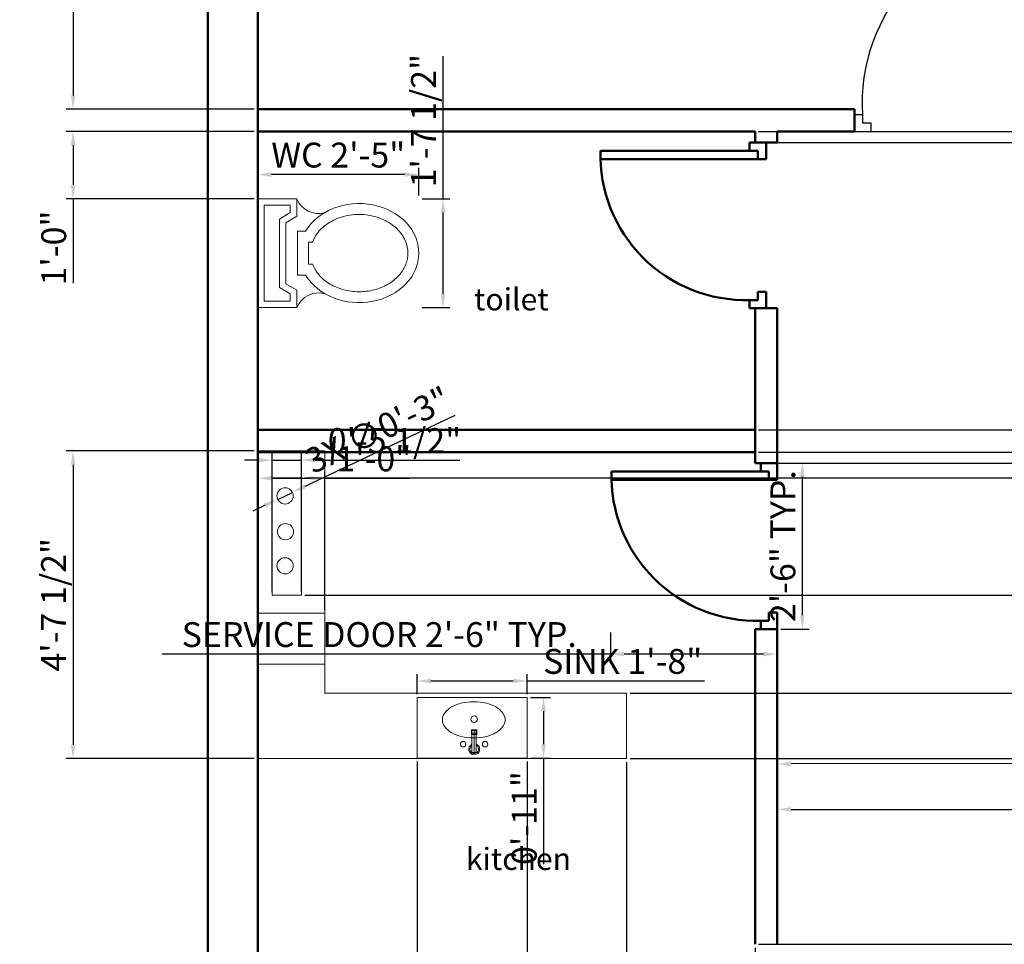
# Model space of a CAD drawing. Units: inches. Extents: x 1253 to 1645, y 2180 to 2698.
# Tile 2 of 5: x 1253 to 1431, y 2363 to 2531. Entities that reach past the tile are written whole.
import ezdxf

# ---------------------------------------------------------------- set-up
doc = ezdxf.new("R2010")
doc.units = ezdxf.units.IN
for name, color, linetype, lineweight in [('A-ANNO-DIMS', 2, 'Continuous', 18), ('A-AREA-IDEN', 7, 'Continuous', 25), ('A-DOOR', 4, 'Continuous', 25), ('A-FLOR-FIXT', 9, 'Continuous', 18), ('wall', 7, 'Continuous', 50)]:
    doc.layers.add(name, color=color, linetype=linetype, lineweight=lineweight)
doc.styles.get("Standard").update_dxf_attribs({"font": 'arial.ttf'})
doc.dimstyles.new('ISO-25', dxfattribs={"dimtxt": 4.5, "dimasz": 2.5, "dimexe": 1.25, "dimexo": 0.625, "dimtad": 1, "dimdec": 1, "dimlunit": 3, "dimtxsty": 'Standard', "dimcen": 4.5, "dimadec": 0, "dimazin": 0, "dimtfac": 1, "dimtdec": 1, "dimtmove": 0, "dimatfit": 3, "dimfxl": 1, "dimarcsym": 0})

# ---------------------------------------------------------------- blocks, each defined once
blk = doc.blocks.new('new block')
for p, q in [((1.5, 1.5), (1.5, 30)), ((3, 0), (3, 30)), ((0, 3), (0, 0)), ((1.5, 3), (0, 3)), ((1.5, 1.5), (1.5, 3)), ((28.5, 1.5), (28.5, 3)), ((28.5, 3), (30, 3)), ((30, 3), (30, 0)), ((0, 0), (3, 0)), ((3, 1.5), (1.5, 1.5)), ((3, 0), (3, 1.5)), ((27, 0), (27, 1.5)), ((27, 1.5), (28.5, 1.5)), ((30, 0), (27, 0))]:
    blk.add_line(p, q)
blk.add_arc((2.25, 3.75), 26.26, 358.3634, 91.6366)
blk = doc.blocks.new('2.6door')
at = {"layer": 'wall'}
blk.add_blockref('new block', (0, 0), dxfattribs=at)
blk = doc.blocks.new('A$C7C8779AE')
for p, q in [((0, 0.7405), (0, 0.5605)), ((0.5, 0.7405), (0, 0.7405)), ((0.5, 0.5605), (0.5, 0.7405)), ((0.47, 0.7105), (0.03, 0.7105)), ((0.03, 0.7105), (0.03, 0.5905)), ((0.47, 0.5905), (0.47, 0.7105)), ((0.093, 0.6405), (0.063, 0.5905)), ((0.093, 0.6405), (0.407, 0.6405)), ((0.437, 0.5905), (0.407, 0.6405)), ((0.03, 0.5905), (0.063, 0.5905)), ((0.11, 0.6105), (0.08, 0.5605)), ((0.11, 0.6105), (0.39, 0.6105)), ((0.42, 0.5605), (0.39, 0.6105)), ((0.437, 0.5905), (0.47, 0.5905)), ((0, 0.5605), (0.08, 0.5605)), ((0.1497, 0.557), (0.1497, 0.5203)), ((0.1497, 0.557), (0.3514, 0.557)), ((0.3514, 0.557), (0.3514, 0.5203)), ((0.42, 0.5605), (0.5, 0.5605)), ((0.1997, 0.507), (0.1997, 0.4879)), ((0.1997, 0.507), (0.3014, 0.507)), ((0.3014, 0.507), (0.3014, 0.4879))]:
    blk.add_line(p, q)
for centre, start, end in [((-0.0386, 0.4613), 344.642, 68.7339), ((0.5386, 0.4613), 111.2661, 195.358)]:
    blk.add_arc(centre, 0.1064, start, end)
blk.add_ellipse((0.2506, 0.2744), major_axis=(0, 0.2744), ratio=0.828948, start_param=0.459479, end_param=5.823706)
blk.add_open_spline([(0.1997, 0.4879), (0.1697, 0.474), (0.1642, 0.4702), (0.1512, 0.4602), (0.1438, 0.4535), (0.1298, 0.4388), (0.1233, 0.4306), (0.1111, 0.4131), (0.1055, 0.4037), (0.0956, 0.3838), (0.0912, 0.3733), (0.0838, 0.3516), (0.0808, 0.3403), (0.0762, 0.3172), (0.0746, 0.3055), (0.073, 0.2817), (0.0729, 0.2698), (0.0743, 0.246), (0.0758, 0.2342), (0.0801, 0.2111), (0.0831, 0.1998), (0.0903, 0.1779), (0.0945, 0.1673), (0.1043, 0.1473), (0.1098, 0.1378), (0.1218, 0.12), (0.1283, 0.1118), (0.1421, 0.0968), (0.1494, 0.09), (0.1646, 0.078), (0.1725, 0.0728), (0.1887, 0.064), (0.1969, 0.0603), (0.2137, 0.0547), (0.2222, 0.0527), (0.2392, 0.0502), (0.2478, 0.0498), (0.2664, 0.0505), (0.2764, 0.052), (0.2963, 0.0573), (0.3061, 0.061), (0.3253, 0.0707), (0.3346, 0.0766), (0.3525, 0.0906), (0.3611, 0.0987), (0.3771, 0.1169), (0.3845, 0.127), (0.3978, 0.1488), (0.4037, 0.1605), (0.4137, 0.1853), (0.4178, 0.1983), (0.424, 0.2251), (0.4261, 0.2389), (0.4282, 0.2668), (0.4283, 0.2809), (0.4262, 0.3088), (0.4241, 0.3226), (0.418, 0.3495), (0.414, 0.3625), (0.404, 0.3873), (0.3982, 0.3991), (0.385, 0.421), (0.3776, 0.4311), (0.3617, 0.4494), (0.3531, 0.4575), (0.3382, 0.4693), (0.3321, 0.4736), (0.3014, 0.4879)], degree=3, knots=[0.459479, 0.459479, 0.459479, 0.459479, 0.567422, 0.567422, 0.720865, 0.720865, 0.874307, 0.874307, 1.02775, 1.02775, 1.181192, 1.181192, 1.334635, 1.334635, 1.488077, 1.488077, 1.64152, 1.64152, 1.794963, 1.794963, 1.948405, 1.948405, 2.101848, 2.101848, 2.25529, 2.25529, 2.408733, 2.408733, 2.562175, 2.562175, 2.715618, 2.715618, 2.86906, 2.86906, 3.022503, 3.022503, 3.175946, 3.175946, 3.356457, 3.356457, 3.536968, 3.536968, 3.717479, 3.717479, 3.89799, 3.89799, 4.078501, 4.078501, 4.259012, 4.259012, 4.439523, 4.439523, 4.620035, 4.620035, 4.800546, 4.800546, 4.981057, 4.981057, 5.161568, 5.161568, 5.342079, 5.342079, 5.52259, 5.52259, 5.703101, 5.703101, 5.823706, 5.823706, 5.823706, 5.823706])
blk = doc.blocks.new('A$C50A015BB')
for p, q in [((0, 0.55), (1, 0.55)), ((0, 0.55), (0, 0)), ((1, 0.55), (1, 0)), ((0.4985, 0.5), (0.5385, 0.5)), ((0.4985, 0.5), (0.4985, 0.3)), ((0.5185, 0.5), (0.5185, 0.3)), ((0.5385, 0.5), (0.5385, 0.3)), ((0.4935, 0.335), (0.4935, 0.295)), ((0.4935, 0.335), (0.5435, 0.335)), ((0.4935, 0.295), (0.5435, 0.295)), ((0.4985, 0.325), (0.5385, 0.325)), ((0.4985, 0.3), (0.5385, 0.3)), ((0.5435, 0.335), (0.5435, 0.295)), ((0, 0), (1, 0)), ((0, 0), (1, 0))]:
    blk.add_line(p, q)
for centre, radius in [((0.4185, 0.424), 0.025), ((0.6185, 0.424), 0.025), ((0.5185, 0.1981), 0.0298)]:
    blk.add_circle(centre, radius)
for centre, radius, start, end in [((0.5201, 0.4703), 0.0497, 291.74253, 244.23308), ((0.5201, 0.4703), 0.0397, 297.63203, 237.02558), ((0.5157, -0.1225), 0.4906, 90, 103.48533), ((0.5157, -0.1225), 0.4906, 76.51467, 90), ((0.4185, 0.1397), 0.2081, 120.06859, 144.41781), ((0.4772, 0.0383), 0.3252, 103.48533, 120.06859), ((0.5543, 0.0383), 0.3252, 59.93141, 76.51467), ((0.613, 0.1397), 0.2081, 35.58219, 59.93141), ((0.3299, 0.2031), 0.0991, 144.41781, 180), ((0.3299, 0.2031), 0.0991, 180, 215.58219), ((0.7016, 0.2031), 0.0991, 0, 35.58219), ((0.7016, 0.2031), 0.0991, 324.41781, 0), ((0.4185, 0.2665), 0.2081, 215.58219, 239.93141), ((0.613, 0.2665), 0.2081, 300.06859, 324.41781), ((0.4772, 0.3679), 0.3252, 239.93141, 256.51467), ((0.5157, 0.5288), 0.4906, 256.51467, 270), ((0.5157, 0.5288), 0.4906, 270, 283.48533), ((0.5543, 0.3679), 0.3252, 283.48533, 300.06859)]:
    blk.add_arc(centre, radius, start, end)
blk = doc.blocks.new('DOOR-SWING-36IN')
for p, q in [((1.5, 1.5), (1.5, 37.5)), ((3, 1.5), (3, 37.5)), ((0, 3), (0, 0)), ((1.5, 3), (0, 3)), ((1.5, 1.5), (1.5, 3)), ((34.5, 1.5), (34.5, 3)), ((34.5, 3), (36, 3)), ((36, 3), (36, 0)), ((3, 1.5), (1.5, 1.5)), ((3, 0), (3, 1.5)), ((33, 0), (33, 1.5)), ((33, 1.5), (34.5, 1.5)), ((0, 0), (3, 0)), ((36, 0), (33, 0))]:
    blk.add_line(p, q)
blk.add_arc((2.25, 5.18), 32.32, 356.1244, 91.3295)
blk = doc.blocks.new('*D20')
at = {"layer": 'A-ANNO-DIMS', "color": 0, "lineweight": -2, "transparency": 16777216}
for p, q in [((1359.74, 2419.72), (1359.74, 2414.57)), ((1389.94, 2419.72), (1389.94, 2414.57)), ((1359.74, 2415.82), (1278.63, 2415.82)), ((1387.44, 2415.82), (1362.24, 2415.82))]:
    blk.add_line(p, q, dxfattribs=at)
at = {"layer": 'A-ANNO-DIMS', "color": 0, "transparency": 16777216}
for points in [[(1362.24, 2416.23), (1362.24, 2415.4), (1359.74, 2415.82)], [(1387.44, 2416.23), (1387.44, 2415.4), (1389.94, 2415.82)]]:
    blk.add_solid(points, dxfattribs=at)
at = {"layer": 'Defpoints', "color": 0, "transparency": 16777216}
for p in [(1359.74, 2420.35), (1389.94, 2420.35), (1359.74, 2415.82)]:
    blk.add_point(p, dxfattribs=at)
at = {"layer": 'A-ANNO-DIMS', "color": 0, "transparency": 16777216, "insert": (1317.93, 2418.77), "char_height": 4.5, "attachment_point": 5}
blk.add_mtext('SERVICE DOOR 2\'-6" TYP.', dxfattribs=at)
blk = doc.blocks.new('*D21')
at = {"layer": 'A-ANNO-DIMS', "color": 0, "lineweight": -2, "transparency": 16777216}
for p, q in [((1390.57, 2450.35), (1395.72, 2450.35)), ((1394.47, 2447.85), (1394.47, 2422.85)), ((1390.57, 2420.35), (1395.72, 2420.35))]:
    blk.add_line(p, q, dxfattribs=at)
at = {"layer": 'A-ANNO-DIMS', "color": 0, "transparency": 16777216}
for points in [[(1394.06, 2447.85), (1394.89, 2447.85), (1394.47, 2450.35)], [(1394.06, 2422.85), (1394.89, 2422.85), (1394.47, 2420.35)]]:
    blk.add_solid(points, dxfattribs=at)
at = {"layer": 'Defpoints', "color": 0, "transparency": 16777216}
for p in [(1389.94, 2450.35), (1389.94, 2420.35), (1394.47, 2420.35)]:
    blk.add_point(p, dxfattribs=at)
at = {"layer": 'A-ANNO-DIMS', "color": 0, "transparency": 16777216, "insert": (1391.55, 2435.35), "char_height": 4.5, "attachment_point": 5, "rotation": 90}
blk.add_mtext('2\'-6" TYP.', dxfattribs=at)
blk = doc.blocks.new('*D22')
at = {"layer": 'A-ANNO-DIMS', "color": 0, "lineweight": -2, "transparency": 16777216}
for p, q in [((1295.94, 2498.78), (1295.94, 2503.78)), ((1325.09, 2498.78), (1325.09, 2503.78)), ((1322.59, 2502.53), (1298.44, 2502.53))]:
    blk.add_line(p, q, dxfattribs=at)
at = {"layer": 'A-ANNO-DIMS', "color": 0, "transparency": 16777216}
for points in [[(1298.44, 2502.95), (1298.44, 2502.11), (1295.94, 2502.53)], [(1322.59, 2502.95), (1322.59, 2502.11), (1325.09, 2502.53)]]:
    blk.add_solid(points, dxfattribs=at)
at = {"layer": 'Defpoints', "color": 0, "transparency": 16777216}
for p in [(1295.94, 2502.53), (1295.94, 2498.16), (1325.09, 2498.16)]:
    blk.add_point(p, dxfattribs=at)
at = {"layer": 'A-ANNO-DIMS', "color": 0, "transparency": 16777216, "insert": (1310.52, 2505.48), "char_height": 4.5, "attachment_point": 5}
blk.add_mtext('WC 2\'-5"', dxfattribs=at)
blk = doc.blocks.new('*D23')
at = {"layer": 'A-ANNO-DIMS', "color": 0, "lineweight": -2, "transparency": 16777216}
for p, q in [((1329.47, 2498.16), (1329.47, 2523.93)), ((1325.72, 2498.16), (1330.72, 2498.16)), ((1329.47, 2480.97), (1329.47, 2495.66)), ((1325.72, 2478.47), (1330.72, 2478.47))]:
    blk.add_line(p, q, dxfattribs=at)
at = {"layer": 'A-ANNO-DIMS', "color": 0, "transparency": 16777216}
for points in [[(1329.05, 2495.66), (1329.88, 2495.66), (1329.47, 2498.16)], [(1329.05, 2480.97), (1329.88, 2480.97), (1329.47, 2478.47)]]:
    blk.add_solid(points, dxfattribs=at)
at = {"layer": 'Defpoints', "color": 0, "transparency": 16777216}
for p in [(1325.09, 2498.16), (1329.47, 2498.16), (1325.09, 2478.47)]:
    blk.add_point(p, dxfattribs=at)
at = {"layer": 'A-ANNO-DIMS', "color": 0, "transparency": 16777216, "insert": (1326.51, 2512.29), "char_height": 4.5, "attachment_point": 5, "rotation": 90}
blk.add_mtext('1\'-7 1/2"', dxfattribs=at)
blk = doc.blocks.new('*D24')
at = {"layer": 'A-ANNO-DIMS', "color": 0, "lineweight": -2, "transparency": 16777216}
for p, q in [((1324.77, 2408.6), (1324.77, 2412.21)), ((1344.68, 2408.6), (1344.68, 2412.21)), ((1327.27, 2410.96), (1342.18, 2410.96)), ((1344.68, 2410.96), (1376.79, 2410.96))]:
    blk.add_line(p, q, dxfattribs=at)
at = {"layer": 'A-ANNO-DIMS', "color": 0, "transparency": 16777216}
for points in [[(1327.27, 2411.38), (1327.27, 2410.55), (1324.77, 2410.96)], [(1342.18, 2411.38), (1342.18, 2410.55), (1344.68, 2410.96)]]:
    blk.add_solid(points, dxfattribs=at)
at = {"layer": 'Defpoints', "color": 0, "transparency": 16777216}
for p in [(1344.68, 2410.96), (1324.77, 2407.98), (1344.68, 2407.98)]:
    blk.add_point(p, dxfattribs=at)
at = {"layer": 'A-ANNO-DIMS', "color": 0, "transparency": 16777216, "insert": (1361.98, 2413.92), "char_height": 4.5, "attachment_point": 5}
blk.add_mtext('SINK 1\'-8"', dxfattribs=at)
blk = doc.blocks.new('*D25')
at = {"layer": 'A-ANNO-DIMS', "color": 0, "lineweight": -2, "transparency": 16777216}
for p, q in [((1345.3, 2407.98), (1348.91, 2407.98)), ((1347.66, 2405.48), (1347.66, 2399.53)), ((1345.3, 2397.03), (1348.91, 2397.03)), ((1347.66, 2397.03), (1347.66, 2377.82))]:
    blk.add_line(p, q, dxfattribs=at)
at = {"layer": 'A-ANNO-DIMS', "color": 0, "transparency": 16777216}
for points in [[(1347.25, 2405.48), (1348.08, 2405.48), (1347.66, 2407.98)], [(1347.25, 2399.53), (1348.08, 2399.53), (1347.66, 2397.03)]]:
    blk.add_solid(points, dxfattribs=at)
at = {"layer": 'Defpoints', "color": 0, "transparency": 16777216}
for p in [(1344.68, 2407.98), (1344.68, 2397.03), (1347.66, 2397.03)]:
    blk.add_point(p, dxfattribs=at)
at = {"layer": 'A-ANNO-DIMS', "color": 0, "transparency": 16777216, "insert": (1344.74, 2386.18), "char_height": 4.5, "attachment_point": 5, "rotation": 90}
blk.add_mtext('0\'-11"', dxfattribs=at)
blk = doc.blocks.new('*D30')
at = {"layer": 'A-ANNO-DIMS', "color": 0, "lineweight": -2, "transparency": 16777216}
for p, q in [((1295.32, 2658.35), (1261.29, 2658.35)), ((1262.54, 2655.85), (1262.54, 2516.85)), ((1295.32, 2514.35), (1261.29, 2514.35))]:
    blk.add_line(p, q, dxfattribs=at)
at = {"layer": 'A-ANNO-DIMS', "color": 0, "transparency": 16777216}
for points in [[(1262.12, 2655.85), (1262.96, 2655.85), (1262.54, 2658.35)], [(1262.12, 2516.85), (1262.96, 2516.85), (1262.54, 2514.35)]]:
    blk.add_solid(points, dxfattribs=at)
at = {"layer": 'Defpoints', "color": 0, "transparency": 16777216}
for p in [(1295.94, 2658.35), (1262.54, 2514.35), (1295.94, 2514.35)]:
    blk.add_point(p, dxfattribs=at)
at = {"layer": 'A-ANNO-DIMS', "color": 0, "transparency": 16777216, "insert": (1259.62, 2586.35), "char_height": 4.5, "attachment_point": 5, "rotation": 90}
blk.add_mtext('12\'-0"', dxfattribs=at)
blk = doc.blocks.new('*D31')
at = {"layer": 'A-ANNO-DIMS', "color": 0, "lineweight": -2, "transparency": 16777216}
for p, q in [((1386.57, 2510.35), (1642.59, 2510.35)), ((1641.34, 2507.85), (1641.34, 2458.85)), ((1386.57, 2456.35), (1642.59, 2456.35))]:
    blk.add_line(p, q, dxfattribs=at)
at = {"layer": 'A-ANNO-DIMS', "color": 0, "transparency": 16777216}
for points in [[(1640.92, 2507.85), (1641.76, 2507.85), (1641.34, 2510.35)], [(1640.92, 2458.85), (1641.76, 2458.85), (1641.34, 2456.35)]]:
    blk.add_solid(points, dxfattribs=at)
at = {"layer": 'Defpoints', "color": 0, "transparency": 16777216}
for p in [(1385.94, 2510.35), (1385.94, 2456.35), (1641.34, 2456.35)]:
    blk.add_point(p, dxfattribs=at)
at = {"layer": 'A-ANNO-DIMS', "color": 0, "transparency": 16777216, "insert": (1638.42, 2483.35), "char_height": 4.5, "attachment_point": 5, "rotation": 90}
blk.add_mtext('4\'-6"', dxfattribs=at)
blk = doc.blocks.new('*D32')
at = {"layer": 'A-ANNO-DIMS', "color": 0, "lineweight": -2, "transparency": 16777216}
for p, q in [((1386.57, 2452.35), (1642.59, 2452.35)), ((1641.34, 2449.85), (1641.34, 2365.85)), ((1386.57, 2363.35), (1642.59, 2363.35))]:
    blk.add_line(p, q, dxfattribs=at)
at = {"layer": 'A-ANNO-DIMS', "color": 0, "transparency": 16777216}
for points in [[(1640.92, 2449.85), (1641.76, 2449.85), (1641.34, 2452.35)], [(1640.92, 2365.85), (1641.76, 2365.85), (1641.34, 2363.35)]]:
    blk.add_solid(points, dxfattribs=at)
at = {"layer": 'Defpoints', "color": 0, "transparency": 16777216}
for p in [(1385.94, 2452.35), (1385.94, 2363.35), (1641.34, 2363.35)]:
    blk.add_point(p, dxfattribs=at)
at = {"layer": 'A-ANNO-DIMS', "color": 0, "transparency": 16777216, "insert": (1638.43, 2407.85), "char_height": 4.5, "attachment_point": 5, "rotation": 90}
blk.add_mtext('7\'-5"', dxfattribs=at)
blk = doc.blocks.new('*D35')
at = {"layer": 'A-ANNO-DIMS', "color": 0, "lineweight": -2, "transparency": 16777216}
for p, q in [((1295.94, 2362.72), (1295.94, 2179.7)), ((1385.94, 2362.72), (1385.94, 2179.7)), ((1298.44, 2180.95), (1383.44, 2180.95))]:
    blk.add_line(p, q, dxfattribs=at)
at = {"layer": 'A-ANNO-DIMS', "color": 0, "transparency": 16777216}
for points in [[(1298.44, 2181.36), (1298.44, 2180.53), (1295.94, 2180.95)], [(1383.44, 2181.36), (1383.44, 2180.53), (1385.94, 2180.95)]]:
    blk.add_solid(points, dxfattribs=at)
at = {"layer": 'Defpoints', "color": 0, "transparency": 16777216}
for p in [(1295.94, 2363.35), (1385.94, 2363.35), (1385.94, 2180.95)]:
    blk.add_point(p, dxfattribs=at)
at = {"layer": 'A-ANNO-DIMS', "color": 0, "transparency": 16777216, "insert": (1340.94, 2183.87), "char_height": 4.5, "attachment_point": 5}
blk.add_mtext('7\'-6"', dxfattribs=at)
blk = doc.blocks.new('*D46')
at = {"layer": 'A-ANNO-DIMS', "color": 0, "lineweight": -2, "transparency": 16777216}
for p, q in [((1641.34, 2512.85), (1641.34, 2515.35)), ((1386.57, 2510.35), (1642.59, 2510.35)), ((1641.34, 2510.35), (1641.34, 2508.35)), ((1386.57, 2508.35), (1642.59, 2508.35)), ((1641.34, 2505.85), (1641.34, 2490.13))]:
    blk.add_line(p, q, dxfattribs=at)
at = {"layer": 'A-ANNO-DIMS', "color": 0, "transparency": 16777216}
for points in [[(1640.92, 2512.85), (1641.76, 2512.85), (1641.34, 2510.35)], [(1640.92, 2505.85), (1641.76, 2505.85), (1641.34, 2508.35)]]:
    blk.add_solid(points, dxfattribs=at)
at = {"layer": 'Defpoints', "color": 0, "transparency": 16777216}
for p in [(1385.94, 2510.35), (1385.94, 2508.35), (1641.34, 2508.35)]:
    blk.add_point(p, dxfattribs=at)
at = {"layer": 'A-ANNO-DIMS', "color": 0, "transparency": 16777216, "insert": (1638.42, 2496.74), "char_height": 4.5, "attachment_point": 5, "rotation": 90}
blk.add_mtext('0\'-2"', dxfattribs=at)
blk = doc.blocks.new('*D47')
at = {"layer": 'A-ANNO-DIMS', "color": 0, "lineweight": -2, "transparency": 16777216}
for p, q in [((1641.34, 2454.85), (1641.34, 2457.35)), ((1386.57, 2452.35), (1642.59, 2452.35)), ((1641.34, 2452.35), (1641.34, 2450.35)), ((1386.57, 2450.35), (1642.59, 2450.35)), ((1641.34, 2447.85), (1641.34, 2432.13))]:
    blk.add_line(p, q, dxfattribs=at)
at = {"layer": 'A-ANNO-DIMS', "color": 0, "transparency": 16777216}
for points in [[(1640.92, 2454.85), (1641.76, 2454.85), (1641.34, 2452.35)], [(1640.92, 2447.85), (1641.76, 2447.85), (1641.34, 2450.35)]]:
    blk.add_solid(points, dxfattribs=at)
at = {"layer": 'Defpoints', "color": 0, "transparency": 16777216}
for p in [(1385.94, 2452.35), (1385.94, 2450.35), (1641.34, 2450.35)]:
    blk.add_point(p, dxfattribs=at)
at = {"layer": 'A-ANNO-DIMS', "color": 0, "transparency": 16777216, "insert": (1638.42, 2438.74), "char_height": 4.5, "attachment_point": 5, "rotation": 90}
blk.add_mtext('0\'-2"', dxfattribs=at)
blk = doc.blocks.new('*D48')
at = {"layer": 'A-ANNO-DIMS', "color": 0, "lineweight": -2, "transparency": 16777216}
for p, q in [((1295.94, 2396.31), (1295.94, 2179.7)), ((1324.77, 2396.41), (1324.77, 2179.7)), ((1298.44, 2180.95), (1322.27, 2180.95))]:
    blk.add_line(p, q, dxfattribs=at)
at = {"layer": 'A-ANNO-DIMS', "color": 0, "transparency": 16777216}
for points in [[(1298.44, 2181.36), (1298.44, 2180.53), (1295.94, 2180.95)], [(1322.27, 2181.36), (1322.27, 2180.53), (1324.77, 2180.95)]]:
    blk.add_solid(points, dxfattribs=at)
at = {"layer": 'Defpoints', "color": 0, "transparency": 16777216}
for p in [(1295.94, 2396.94), (1324.77, 2397.03), (1324.77, 2180.95)]:
    blk.add_point(p, dxfattribs=at)
at = {"layer": 'A-ANNO-DIMS', "color": 0, "transparency": 16777216, "insert": (1310.36, 2183.87), "char_height": 4.5, "attachment_point": 5}
blk.add_mtext('2\'-5"', dxfattribs=at)
blk = doc.blocks.new('*D49')
at = {"layer": 'A-ANNO-DIMS', "color": 0, "lineweight": -2, "transparency": 16777216}
for p, q in [((1295.32, 2452.55), (1261.29, 2452.55)), ((1262.54, 2450.05), (1262.54, 2399.44)), ((1295.32, 2396.94), (1261.29, 2396.94))]:
    blk.add_line(p, q, dxfattribs=at)
at = {"layer": 'A-ANNO-DIMS', "color": 0, "transparency": 16777216}
for points in [[(1262.12, 2450.05), (1262.96, 2450.05), (1262.54, 2452.55)], [(1262.12, 2399.44), (1262.96, 2399.44), (1262.54, 2396.94)]]:
    blk.add_solid(points, dxfattribs=at)
at = {"layer": 'Defpoints', "color": 0, "transparency": 16777216}
for p in [(1295.94, 2452.55), (1262.54, 2396.94), (1295.94, 2396.94)]:
    blk.add_point(p, dxfattribs=at)
at = {"layer": 'A-ANNO-DIMS', "color": 0, "transparency": 16777216, "insert": (1259.59, 2424.74), "char_height": 4.5, "attachment_point": 5, "rotation": 90}
blk.add_mtext('4\'-7 1/2"', dxfattribs=at)
blk = doc.blocks.new('*D50')
at = {"layer": 'A-ANNO-DIMS', "color": 0, "lineweight": -2, "transparency": 16777216}
for p, q in [((1363.3, 2408.78), (1642.59, 2408.78)), ((1641.34, 2406.28), (1641.34, 2399.44)), ((1363.3, 2396.94), (1642.59, 2396.94)), ((1641.34, 2396.94), (1641.34, 2381.65))]:
    blk.add_line(p, q, dxfattribs=at)
at = {"layer": 'A-ANNO-DIMS', "color": 0, "transparency": 16777216}
for points in [[(1640.92, 2406.28), (1641.76, 2406.28), (1641.34, 2408.78)], [(1640.92, 2399.44), (1641.76, 2399.44), (1641.34, 2396.94)]]:
    blk.add_solid(points, dxfattribs=at)
at = {"layer": 'Defpoints', "color": 0, "transparency": 16777216}
for p in [(1362.68, 2408.78), (1362.68, 2396.94), (1641.34, 2396.94)]:
    blk.add_point(p, dxfattribs=at)
at = {"layer": 'A-ANNO-DIMS', "color": 0, "transparency": 16777216, "insert": (1638.42, 2388.04), "char_height": 4.5, "attachment_point": 5, "rotation": 90}
blk.add_mtext('1\'-0"', dxfattribs=at)
blk = doc.blocks.new('*D51')
at = {"layer": 'A-ANNO-DIMS', "color": 0, "lineweight": -2, "transparency": 16777216}
for p, q in [((1295.32, 2510.35), (1261.29, 2510.35)), ((1262.54, 2507.85), (1262.54, 2500.66)), ((1295.32, 2498.16), (1261.29, 2498.16)), ((1262.54, 2498.16), (1262.54, 2482.87))]:
    blk.add_line(p, q, dxfattribs=at)
at = {"layer": 'A-ANNO-DIMS', "color": 0, "transparency": 16777216}
for points in [[(1262.12, 2507.85), (1262.96, 2507.85), (1262.54, 2510.35)], [(1262.12, 2500.66), (1262.96, 2500.66), (1262.54, 2498.16)]]:
    blk.add_solid(points, dxfattribs=at)
at = {"layer": 'Defpoints', "color": 0, "transparency": 16777216}
for p in [(1295.94, 2510.35), (1262.54, 2498.16), (1295.94, 2498.16)]:
    blk.add_point(p, dxfattribs=at)
at = {"layer": 'A-ANNO-DIMS', "color": 0, "transparency": 16777216, "insert": (1259.62, 2489.26), "char_height": 4.5, "attachment_point": 5, "rotation": 90}
blk.add_mtext('1\'-0"', dxfattribs=at)
blk = doc.blocks.new('*D52')
at = {"layer": 'A-ANNO-DIMS', "color": 0, "lineweight": -2, "transparency": 16777216}
for p, q in [((1344.68, 2396.41), (1344.68, 2179.7)), ((1362.68, 2396.31), (1362.68, 2179.7)), ((1360.18, 2180.95), (1347.18, 2180.95))]:
    blk.add_line(p, q, dxfattribs=at)
at = {"layer": 'A-ANNO-DIMS', "color": 0, "transparency": 16777216}
for points in [[(1347.18, 2181.36), (1347.18, 2180.53), (1344.68, 2180.95)], [(1360.18, 2181.36), (1360.18, 2180.53), (1362.68, 2180.95)]]:
    blk.add_solid(points, dxfattribs=at)
at = {"layer": 'Defpoints', "color": 0, "transparency": 16777216}
for p in [(1344.68, 2397.03), (1362.68, 2396.94), (1344.68, 2180.95)]:
    blk.add_point(p, dxfattribs=at)
at = {"layer": 'A-ANNO-DIMS', "color": 0, "transparency": 16777216, "insert": (1353.68, 2183.87), "char_height": 4.5, "attachment_point": 5}
blk.add_mtext('1\'-6"', dxfattribs=at)
blk = doc.blocks.new('*D53')
at = {"layer": 'A-ANNO-DIMS', "color": 0, "lineweight": -2, "transparency": 16777216}
for p, q in [((1295.94, 2423.85), (1295.94, 2448.87)), ((1308.06, 2423.85), (1308.06, 2448.87)), ((1298.44, 2447.62), (1305.56, 2447.62)), ((1308.06, 2447.62), (1323.35, 2447.62))]:
    blk.add_line(p, q, dxfattribs=at)
at = {"layer": 'A-ANNO-DIMS', "color": 0, "transparency": 16777216}
for points in [[(1298.44, 2448.04), (1298.44, 2447.21), (1295.94, 2447.62)], [(1305.56, 2448.04), (1305.56, 2447.21), (1308.06, 2447.62)]]:
    blk.add_solid(points, dxfattribs=at)
at = {"layer": 'Defpoints', "color": 0, "transparency": 16777216}
for p in [(1308.06, 2447.62), (1295.94, 2423.22), (1308.06, 2423.22)]:
    blk.add_point(p, dxfattribs=at)
at = {"layer": 'A-ANNO-DIMS', "color": 0, "transparency": 16777216, "insert": (1316.95, 2450.55), "char_height": 4.5, "attachment_point": 5}
blk.add_mtext('1\'-0"', dxfattribs=at)
blk = doc.blocks.new('*D54')
at = {"layer": 'A-ANNO-DIMS', "color": 0, "lineweight": -2, "transparency": 16777216}
for p, q in [((1298.54, 2427.13), (1298.54, 2452.15)), ((1303.84, 2427.13), (1303.84, 2452.15)), ((1296.04, 2450.9), (1293.54, 2450.9)), ((1298.54, 2450.9), (1303.84, 2450.9)), ((1306.34, 2450.9), (1332.54, 2450.9))]:
    blk.add_line(p, q, dxfattribs=at)
at = {"layer": 'A-ANNO-DIMS', "color": 0, "transparency": 16777216}
for points in [[(1296.04, 2451.32), (1296.04, 2450.49), (1298.54, 2450.9)], [(1306.34, 2451.32), (1306.34, 2450.49), (1303.84, 2450.9)]]:
    blk.add_solid(points, dxfattribs=at)
at = {"layer": 'Defpoints', "color": 0, "transparency": 16777216}
for p in [(1303.84, 2450.9), (1298.54, 2426.5), (1303.84, 2426.5)]:
    blk.add_point(p, dxfattribs=at)
at = {"layer": 'A-ANNO-DIMS', "color": 0, "transparency": 16777216, "insert": (1320.69, 2453.85), "char_height": 4.5, "attachment_point": 5}
blk.add_mtext('0\'-5 1/2"', dxfattribs=at)
blk = doc.blocks.new('*D55')
at = {"layer": 'A-ANNO-DIMS', "color": 0, "lineweight": -2, "transparency": 16777216}
for p, q in [((1304.46, 2447.68), (1642.59, 2447.68)), ((1641.34, 2445.18), (1641.34, 2429)), ((1304.46, 2426.5), (1642.59, 2426.5))]:
    blk.add_line(p, q, dxfattribs=at)
at = {"layer": 'A-ANNO-DIMS', "color": 0, "transparency": 16777216}
for points in [[(1640.92, 2445.18), (1641.76, 2445.18), (1641.34, 2447.68)], [(1640.92, 2429), (1641.76, 2429), (1641.34, 2426.5)]]:
    blk.add_solid(points, dxfattribs=at)
at = {"layer": 'Defpoints', "color": 0, "transparency": 16777216}
for p in [(1303.84, 2447.68), (1303.84, 2426.5), (1641.34, 2426.5)]:
    blk.add_point(p, dxfattribs=at)
at = {"layer": 'A-ANNO-DIMS', "color": 0, "transparency": 16777216, "insert": (1638.42, 2437.09), "char_height": 4.5, "attachment_point": 5, "rotation": 90}
blk.add_mtext('1\'-9"', dxfattribs=at)
blk = doc.blocks.new('*D56')
at = {"layer": 'A-ANNO-DIMS', "color": 0, "lineweight": -2, "transparency": 16777216}
for p, q in [((1389.94, 2419.72), (1390, 2394.7)), ((1489.14, 2419.94), (1489.19, 2394.91)), ((1486.69, 2396.16), (1392.5, 2395.95))]:
    blk.add_line(p, q, dxfattribs=at)
at = {"layer": 'A-ANNO-DIMS', "color": 0, "transparency": 16777216}
for points in [[(1392.49, 2396.37), (1392.5, 2395.54), (1390, 2395.95)], [(1486.69, 2396.58), (1486.69, 2395.74), (1489.19, 2396.16)]]:
    blk.add_solid(points, dxfattribs=at)
at = {"layer": 'Defpoints', "color": 0, "transparency": 16777216}
for p in [(1389.94, 2420.35), (1489.14, 2420.56), (1390, 2395.95)]:
    blk.add_point(p, dxfattribs=at)
at = {"layer": 'A-ANNO-DIMS', "color": 0, "transparency": 16777216, "insert": (1439.59, 2398.98), "char_height": 4.5, "attachment_point": 5, "rotation": 0.126}
blk.add_mtext('8\'-3"', dxfattribs=at)
blk = doc.blocks.new('*D58')
at = {"layer": 'A-ANNO-DIMS', "color": 0, "lineweight": -2, "transparency": 16777216}
for p, q in [((1389.94, 2363.97), (1389.94, 2389)), ((1607.94, 2363.97), (1607.94, 2389)), ((1392.44, 2387.75), (1605.44, 2387.75))]:
    blk.add_line(p, q, dxfattribs=at)
at = {"layer": 'A-ANNO-DIMS', "color": 0, "transparency": 16777216}
for points in [[(1392.44, 2388.16), (1392.44, 2387.33), (1389.94, 2387.75)], [(1605.44, 2388.16), (1605.44, 2387.33), (1607.94, 2387.75)]]:
    blk.add_solid(points, dxfattribs=at)
at = {"layer": 'Defpoints', "color": 0, "transparency": 16777216}
for p in [(1607.94, 2387.75), (1389.94, 2363.35), (1607.94, 2363.35)]:
    blk.add_point(p, dxfattribs=at)
at = {"layer": 'A-ANNO-DIMS', "color": 0, "transparency": 16777216, "insert": (1498.94, 2390.67), "char_height": 4.5, "attachment_point": 5}
blk.add_mtext('18\'-2"', dxfattribs=at)
blk = doc.blocks.new('*D64')
at = {"layer": 'A-ANNO-DIMS', "color": 0, "lineweight": -2, "transparency": 16777216}
for p, q in [((1331.63, 2458.97), (1304.48, 2446.13)), ((1299.57, 2443.8), (1302.22, 2445.06)), ((1297.31, 2442.73), (1295.05, 2441.67))]:
    blk.add_line(p, q, dxfattribs=at)
at = {"layer": 'A-ANNO-DIMS', "color": 0, "transparency": 16777216}
for points in [[(1304.3, 2446.5), (1304.66, 2445.75), (1302.22, 2445.06)], [(1297.13, 2443.11), (1297.49, 2442.36), (1299.57, 2443.8)]]:
    blk.add_solid(points, dxfattribs=at)
at = {"layer": 'Defpoints', "color": 0, "transparency": 16777216}
for p in [(1302.22, 2445.06), (1299.57, 2443.8)]:
    blk.add_point(p, dxfattribs=at)
at = {"layer": 'A-ANNO-DIMS', "color": 0, "transparency": 16777216, "insert": (1317.88, 2455.84), "char_height": 4.5, "attachment_point": 5, "rotation": 25.3162}
blk.add_mtext('3X ∅0\'-3"', dxfattribs=at)

msp = doc.modelspace()

# ---------------------------------------------------------------- linework, layer by layer
at = {"layer": 'A-FLOR-FIXT'}
for p, q in [((1295.94, 2452.55), (1308.06, 2452.55)), ((1295.94, 2396.94), (1295.94, 2452.55)), ((1308.06, 2452.55), (1308.06, 2408.78)), ((1362.68, 2408.78), (1308.06, 2408.78)), ((1362.68, 2396.94), (1362.68, 2408.78)), ((1295.94, 2396.94), (1362.68, 2396.94))]:
    msp.add_line(p, q, dxfattribs=at)
for points in [[(1298.54, 2447.68), (1303.84, 2447.68), (1303.84, 2426.5), (1298.54, 2426.5)], [(1295.94, 2423.22), (1308.06, 2423.22), (1308.06, 2413.98), (1295.94, 2413.98)]]:
    msp.add_lwpolyline(points, close=True, dxfattribs=at)
for centre in [(1300.9, 2444.43), (1300.97, 2437.96), (1300.9, 2431.79)]:
    msp.add_circle(centre, 1.47, dxfattribs=at)
at = {"layer": 'wall'}
for p, q in [((1286.94, 2667.35), (1286.94, 2205.35)), ((1295.94, 2658.35), (1295.94, 2214.35)), ((1403.94, 2514.35), (1295.94, 2514.35)), ((1403.94, 2514.35), (1403.94, 2510.35)), ((1385.94, 2510.35), (1295.94, 2510.35)), ((1385.94, 2510.35), (1385.94, 2508.35)), ((1389.94, 2510.35), (1389.94, 2508.35)), ((1403.94, 2510.35), (1389.94, 2510.35)), ((1385.94, 2508.35), (1389.94, 2508.35)), ((1385.94, 2478.35), (1389.94, 2478.35)), ((1385.94, 2478.35), (1385.94, 2450.35)), ((1389.94, 2478.35), (1389.94, 2450.35)), ((1385.94, 2456.35), (1295.94, 2456.35)), ((1385.94, 2452.35), (1295.94, 2452.35)), ((1385.94, 2450.35), (1389.94, 2450.35)), ((1385.94, 2420.35), (1389.94, 2420.35)), ((1385.94, 2420.35), (1385.94, 2363.35)), ((1389.94, 2420.35), (1389.94, 2363.35))]:
    msp.add_line(p, q, dxfattribs=at)

# ---------------------------------------------------------------- block references
at = {"layer": 'A-DOOR', "extrusion": (0, 0, -1), "zscale": -1}
msp.add_blockref('DOOR-SWING-36IN', (-1439.94, 2510.35), dxfattribs=at)
at = {"layer": 'A-DOOR', "xscale": -1, "rotation": 90}
for p in [(1387.94, 2508.35), (1389.94, 2450.35)]:
    msp.add_blockref('2.6door', p, dxfattribs=at)
at = {"layer": 'A-FLOR-FIXT'}
for name, p, xscale, yscale, zscale, rotation in [('A$C7C8779AE', (1325.09, 2478.47), 39.37007874015748, 39.37007874015748, 39.37007874015748, 90), ('A$C50A015BB', (1324.77, 2407.98), -19.90433800274748, 19.90433800274748, 19.90433800274748, 180)]:
    msp.add_blockref(name, p, dxfattribs=dict(at, xscale=xscale, yscale=yscale, zscale=zscale, rotation=rotation))

# ---------------------------------------------------------------- texts
at = {"layer": 'A-AREA-IDEN', "char_height": 4, "attachment_point": 1}
for s, insert in [('toilet', (1335.08, 2481.98)), ('kitchen', (1333.61, 2380.79))]:
    msp.add_mtext_dynamic_manual_height_columns(s, width=71.3777, gutter_width=12.5, heights=[0], dxfattribs=dict(at, insert=insert))

# ---------------------------------------------------------------- dimensions: what is measured, and where the dimension line sits
at = {"layer": 'A-ANNO-DIMS'}
for base, p1, p2, angle, picture, middle in [((1262.54, 2514.35), (1295.94, 2658.35), (1295.94, 2514.35), 90, '*D30', (1259.62, 2586.35)), ((1329.47, 2498.16), (1325.09, 2478.47), (1325.09, 2498.16), 90, '*D23', (1326.51, 2512.29)), ((1641.34, 2508.35), (1385.94, 2510.35), (1385.94, 2508.35), 90, '*D46', (1638.42, 2496.74)), ((1262.54, 2498.16), (1295.94, 2510.35), (1295.94, 2498.16), 90, '*D51', (1259.62, 2489.26)), ((1641.34, 2456.35), (1385.94, 2510.35), (1385.94, 2456.35), 90, '*D31', (1638.42, 2483.35)), ((1641.34, 2450.35), (1385.94, 2452.35), (1385.94, 2450.35), 90, '*D47', (1638.42, 2438.74)), ((1262.54, 2396.94), (1295.94, 2452.55), (1295.94, 2396.94), 90, '*D49', (1259.59, 2424.74)), ((1641.34, 2363.35), (1385.94, 2452.35), (1385.94, 2363.35), 90, '*D32', (1638.43, 2407.85)), ((1641.34, 2426.5), (1303.84, 2447.68), (1303.84, 2426.5), 90, '*D55', (1638.42, 2437.09)), ((1390, 2395.95), (1489.14, 2420.56), (1389.94, 2420.35), 180.126, '*D56', (1439.59, 2398.98)), ((1641.34, 2396.94), (1362.68, 2408.78), (1362.68, 2396.94), 90, '*D50', (1638.42, 2388.04)), ((1347.6643, 2397.0308), (1344.6787, 2407.9782), (1344.6787, 2397.0308), 270, '*D25', (1344.7417, 2386.1766))]:
    dim = msp.add_linear_dim(base=base, p1=p1, p2=p2, angle=angle, dimstyle='ISO-25', override={"dimdec": 1, "dimlfac": 1, "dimrnd": 0, "dimzin": 1, "dimdsep": 46, "dimlunit": 4, "dimfrac": 2}, dxfattribs=at)
    dim.commit()
    dim.dimension.update_dxf_attribs({"geometry": picture, "text_midpoint": middle})
for base, p1, p2, angle, text, picture, middle in [((1295.9414, 2502.5292), (1325.0934, 2498.1564), (1295.9414, 2498.1564), 180, 'WC <>', '*D22', (1310.5174, 2505.4809)), ((1394.47, 2420.35), (1389.94, 2450.35), (1389.94, 2420.35), 270, '<> TYP.', '*D21', (1391.55, 2435.35)), ((1359.74, 2415.82), (1389.94, 2420.35), (1359.74, 2420.35), 180, 'SERVICE DOOR <> TYP.', '*D20', (1317.93, 2418.77))]:
    dim = msp.add_linear_dim(base=base, p1=p1, p2=p2, angle=angle, text=text, dimstyle='ISO-25', override={"dimdec": 1, "dimlfac": 1, "dimrnd": 0, "dimzin": 1, "dimdsep": 46, "dimlunit": 4, "dimfrac": 2}, dxfattribs=at)
    dim.commit()
    dim.dimension.update_dxf_attribs({"geometry": picture, "text_midpoint": middle})
dim = msp.add_diameter_dim_2p(p1=(1299.57, 2443.8), p2=(1302.22, 2445.06), text='3X <>', dimstyle='ISO-25', override={"dimdec": 1, "dimlfac": 1, "dimrnd": 0, "dimzin": 1, "dimdsep": 46, "dimlunit": 4, "dimfrac": 2}, dxfattribs=at)
dim.commit()
dim.dimension.update_dxf_attribs({"geometry": '*D64', "text_midpoint": (1319.18, 2453.08), "dimtype": 163})
for base, p1, p2, picture, middle in [((1303.84, 2450.9), (1298.54, 2426.5), (1303.84, 2426.5), '*D54', (1320.69, 2453.85)), ((1308.06, 2447.62), (1295.94, 2423.22), (1308.06, 2423.22), '*D53', (1316.95, 2450.55)), ((1324.77, 2180.95), (1295.94, 2396.94), (1324.77, 2397.03), '*D48', (1310.36, 2183.87)), ((1344.68, 2180.95), (1362.68, 2396.94), (1344.68, 2397.03), '*D52', (1353.68, 2183.87)), ((1607.94, 2387.75), (1389.94, 2363.35), (1607.94, 2363.35), '*D58', (1498.94, 2390.67)), ((1385.94, 2180.95), (1295.94, 2363.35), (1385.94, 2363.35), '*D35', (1340.94, 2183.87))]:
    dim = msp.add_linear_dim(base=base, p1=p1, p2=p2, dimstyle='ISO-25', override={"dimdec": 1, "dimlfac": 1, "dimrnd": 0, "dimzin": 1, "dimdsep": 46, "dimlunit": 4, "dimfrac": 2}, dxfattribs=at)
    dim.commit()
    dim.dimension.update_dxf_attribs({"geometry": picture, "text_midpoint": middle})
dim = msp.add_linear_dim(base=(1344.68, 2410.96), p1=(1324.77, 2407.98), p2=(1344.68, 2407.98), text='SINK <>', dimstyle='ISO-25', override={"dimdec": 1, "dimlfac": 1, "dimrnd": 0, "dimzin": 1, "dimdsep": 46, "dimlunit": 4, "dimfrac": 2}, dxfattribs=at)
dim.commit()
dim.dimension.update_dxf_attribs({"geometry": '*D24', "text_midpoint": (1361.98, 2413.92)})

doc.saveas('drawing.dxf')
